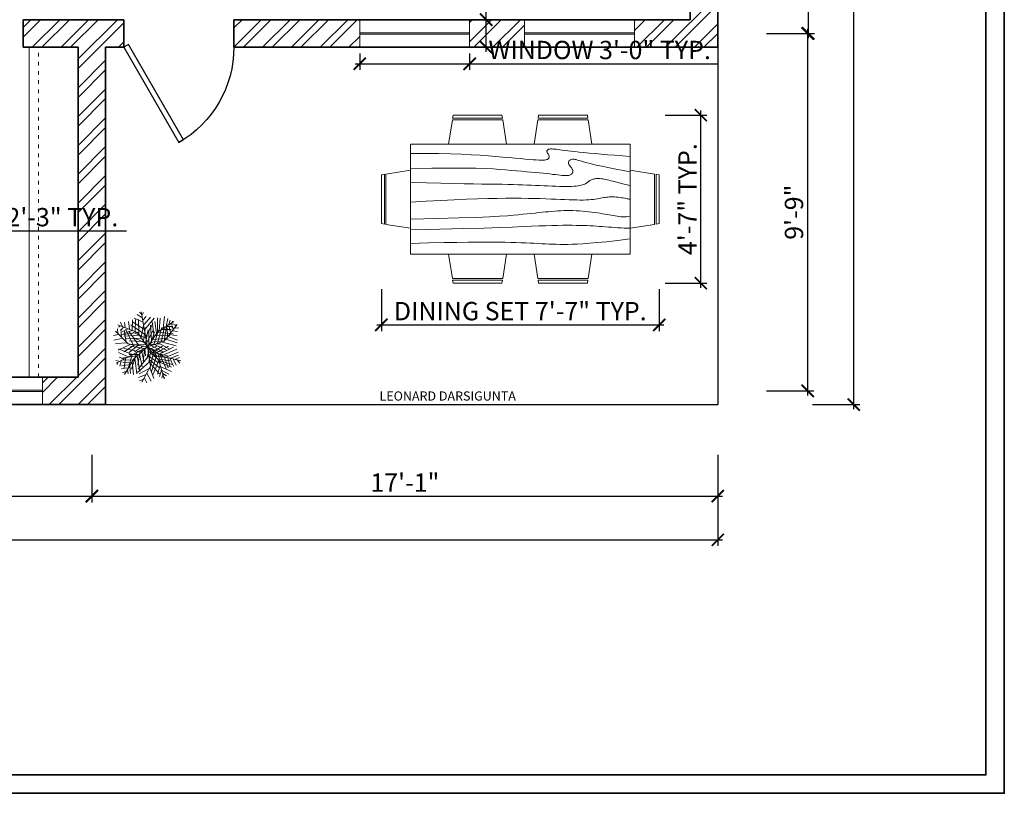
# Model space of a CAD drawing. Units: inches. Extents: x 163 to 947, y 159 to 804.
# Tile 4 of 5: x 625 to 947, y 159 to 412. Entities that reach past the tile are written whole.
import ezdxf

# ---------------------------------------------------------------- set-up
doc = ezdxf.new("R2010")
doc.units = ezdxf.units.IN
doc.linetypes.add('ACAD_ISO03W100', pattern=[30, 12, -18])
for name, color, linetype, lineweight in [('A-ANNO-TEXT', 7, 'Continuous', 18), ('A-ANNO-TTLB', 7, 'Continuous', 35), ('A-FLOR-CASE', 7, 'Continuous', 18), ('A-FLOR-CASE-OVHD', 7, 'ACAD_ISO03W100', 18), ('A-FLOR-OTLN', 7, 'Continuous', 25), ('Dimensions', 7, 'Continuous', 18), ('Doors', 160, 'Continuous', 25), ('Furniture', 40, 'Continuous', 18), ('Greenary  Plants', 100, 'Continuous', 13), ('Wall Hatch', 214, 'Continuous', 13), ('Walls', 222, 'Continuous', 35), ('Windows', 132, 'Continuous', 18)]:
    doc.layers.add(name, color=color, linetype=linetype, lineweight=lineweight)
doc.styles.get("Standard").update_dxf_attribs({"font": 'arial.ttf'})
doc.dimstyles.new('ISO-25', dxfattribs={"dimtxt": 6, "dimasz": 4, "dimexe": 2, "dimexo": 2, "dimtad": 1, "dimdec": 1, "dimlunit": 3, "dimtxsty": 'Standard', "dimblk": 'ARCHTICK', "dimcen": 0, "dimdle": 1.5, "dimadec": 0, "dimazin": 0, "dimtfac": 1, "dimtdec": 1, "dimtmove": 0, "dimatfit": 3, "dimfxl": 13.5, "dimfxlon": 1, "dimarcsym": 0})

# ---------------------------------------------------------------- blocks, each defined once
blk = doc.blocks.new('_ArchTick')
at = {"color": 0, "linetype": 'ByBlock', "const_width": 0.15}
blk.add_lwpolyline([(-0.5, -0.5), (0.5, 0.5)], dxfattribs=at)
blk = doc.blocks.new('*D10')
at = {"layer": 'Dimensions', "color": 0, "lineweight": -2, "transparency": 16777216}
for p, q in [((869.75, 517.32), (885.25, 517.32)), ((883.25, 518.82), (883.25, 405.78)), ((869.75, 407.28), (885.25, 407.28))]:
    blk.add_line(p, q, dxfattribs=at)
at = {"layer": 'Dimensions', "color": 0, "lineweight": -2, "transparency": 16777216, "xscale": 4, "yscale": 4, "zscale": 4}
for p, rotation in [((883.25, 517.32), 90), ((883.25, 407.28), 270)]:
    blk.add_blockref('_ArchTick', p, dxfattribs=dict(at, rotation=rotation))
at = {"layer": 'Dimensions', "color": 0, "transparency": 16777216, "insert": (879.57, 462.3), "char_height": 6, "attachment_point": 5, "rotation": 90}
blk.add_mtext('9\'-2"', dxfattribs=at)
blk = doc.blocks.new('*D11')
at = {"layer": 'Dimensions', "color": 0, "lineweight": -2, "transparency": 16777216}
for p, q in [((869.53, 407.28), (885.03, 407.28)), ((883.03, 408.78), (883.03, 288.78)), ((869.53, 290.28), (885.03, 290.28))]:
    blk.add_line(p, q, dxfattribs=at)
at = {"layer": 'Dimensions', "color": 0, "lineweight": -2, "transparency": 16777216, "xscale": 4, "yscale": 4, "zscale": 4}
for p, rotation in [((883.03, 407.28), 90), ((883.03, 290.28), 270)]:
    blk.add_blockref('_ArchTick', p, dxfattribs=dict(at, rotation=rotation))
at = {"layer": 'Dimensions', "color": 0, "transparency": 16777216, "insert": (879.34, 348.78), "char_height": 6, "attachment_point": 5, "rotation": 90}
blk.add_mtext('9\'-9"', dxfattribs=at)
blk = doc.blocks.new('*D13')
at = {"layer": 'Dimensions', "color": 0, "lineweight": -2, "transparency": 16777216}
for p, q in [((443.62, 269.28), (443.62, 253.78)), ((648.62, 269.28), (648.62, 253.78)), ((442.12, 255.78), (650.12, 255.78))]:
    blk.add_line(p, q, dxfattribs=at)
at = {"layer": 'Dimensions', "color": 0, "lineweight": -2, "transparency": 16777216, "xscale": 4, "yscale": 4, "zscale": 4, "rotation": 180}
blk.add_blockref('_ArchTick', (443.62, 255.78), dxfattribs=at)
at = {"layer": 'Dimensions', "color": 0, "lineweight": -2, "transparency": 16777216, "xscale": 4, "yscale": 4, "zscale": 4}
blk.add_blockref('_ArchTick', (648.62, 255.78), dxfattribs=at)
at = {"layer": 'Dimensions', "color": 0, "transparency": 16777216, "insert": (546.12, 259.41), "char_height": 6, "attachment_point": 5}
blk.add_mtext('17\'-1"', dxfattribs=at)
blk = doc.blocks.new('*D14')
at = {"layer": 'Dimensions', "color": 0, "lineweight": -2, "transparency": 16777216}
for p, q in [((648.62, 269.35), (648.62, 253.85)), ((853.62, 269.35), (853.62, 253.85)), ((647.12, 255.85), (855.12, 255.85))]:
    blk.add_line(p, q, dxfattribs=at)
at = {"layer": 'Dimensions', "color": 0, "lineweight": -2, "transparency": 16777216, "xscale": 4, "yscale": 4, "zscale": 4, "rotation": 180}
blk.add_blockref('_ArchTick', (648.62, 255.85), dxfattribs=at)
at = {"layer": 'Dimensions', "color": 0, "lineweight": -2, "transparency": 16777216, "xscale": 4, "yscale": 4, "zscale": 4}
blk.add_blockref('_ArchTick', (853.62, 255.85), dxfattribs=at)
at = {"layer": 'Dimensions', "color": 0, "transparency": 16777216, "insert": (751.12, 259.48), "char_height": 6, "attachment_point": 5}
blk.add_mtext('17\'-1"', dxfattribs=at)
blk = doc.blocks.new('*U23')
for p, q in [((-36, 0), (-36, 6)), ((0, 0), (0, 6))]:
    blk.add_line(p, q)
blk.add_lwpolyline([(0, 0), (-18, -31.18), (-19.52, -30.3), (-1.52, 0.88)], close=True)
blk.add_arc((0, 0), 36, 180, 240)
blk = doc.blocks.new('Dining Set - 36 x 72 in.')
for p, q in [((-22.2343, 26.00059), (-23.4847, 17.99762)), ((-22.2304, 26), (-5.7608, 26)), ((-22, 27.5), (-22.1562, 26.50042)), ((-5.8416, 26.5), (-22.1534, 26.5)), ((-22, 27.5), (-6, 27.5)), ((-5.8437, 26.49966), (-6, 27.5)), ((-4.5152, 17.99762), (-5.7655, 25.99926)), ((5.7657, 26.00059), (4.5153, 17.99762)), ((5.7696, 26), (22.2392, 26)), ((6, 27.5), (5.8438, 26.50042)), ((22.1584, 26.5), (5.8466, 26.5)), ((6, 27.5), (22, 27.5)), ((22.1563, 26.49966), (22, 27.5)), ((23.4848, 17.99762), (22.2345, 25.99926)), ((36, 18), (-36, 18)), ((-36, 18), (-36, -18)), ((36, -18), (36, 18)), ((-45.5, 8), (-44.5004, 8.15617)), ((-45.5, 8), (-45.5, -8)), ((-44.5, -8.15843), (-44.5, 8.15338)), ((-44.0006, 8.23428), (-35.9976, 9.48474)), ((-44, 8.23041), (-44, -8.23915)), ((44.0006, 8.23428), (35.9976, 9.48474)), ((44, 8.23041), (44, -8.23915)), ((44.5, -8.15843), (44.5, 8.15338)), ((45.5, 8), (44.5005, 8.15617)), ((45.5, 8), (45.5, -8)), ((-44.4997, -8.15631), (-45.5, -8)), ((-35.9976, -9.48476), (-43.9993, -8.2345)), ((35.9976, -9.48476), (43.9993, -8.2345)), ((44.4997, -8.15631), (45.5, -8)), ((-36, -18), (36, -18)), ((-22.2343, -26.0006), (-23.4847, -17.99762)), ((-4.5152, -17.99762), (-5.7655, -25.99928)), ((5.7657, -26.0006), (4.5153, -17.99762)), ((23.4848, -17.99762), (22.2345, -25.99928)), ((-22.2304, -26), (-5.7608, -26)), ((-22, -27.5), (-22.1562, -26.50044)), ((-5.8416, -26.5), (-22.1534, -26.5)), ((-22, -27.5), (-6, -27.5)), ((-5.8437, -26.49967), (-6, -27.5)), ((5.7696, -26), (22.2392, -26)), ((6, -27.5), (5.8438, -26.50044)), ((22.1584, -26.5), (5.8466, -26.5)), ((6, -27.5), (22, -27.5)), ((22.1563, -26.49967), (22, -27.5))]:
    blk.add_line(p, q)
for points in [[(-36, 15), (-31.1772, 14.97754), (-26.8079, 14.91406), (-22.8538, 14.81543), (-19.276, 14.6875), (-16.0362, 14.53613), (-13.0957, 14.36718), (-10.4159, 14.18652), (-7.9583, 14), (-5.6904, 13.81315), (-3.6035, 13.63021), (-1.6954, 13.45508), (0.0365, 13.29166), (1.5945, 13.14388), (2.9811, 13.01562), (4.1988, 12.9108), (5.25, 12.83333), (6.1393, 12.78613), (6.8802, 12.76823), (7.4883, 12.77767), (7.9792, 12.8125), (8.3685, 12.87077), (8.6719, 12.95052), (8.9049, 13.0498), (9.0833, 13.16666), (9.2205, 13.29899), (9.3216, 13.44401), (9.3895, 13.59879), (9.4271, 13.76041), (9.4373, 13.92594), (9.4232, 14.09245), (9.3875, 14.257), (9.3333, 14.41666), (9.2638, 14.56917), (9.1836, 14.71484), (9.0975, 14.85465), (9.0104, 14.98958), (8.9272, 15.1206), (8.8529, 15.2487), (8.7922, 15.37483), (8.75, 15.5), (8.7305, 15.62467), (8.7344, 15.74739), (8.7617, 15.86621), (8.8125, 15.97916), (8.8867, 16.08431), (8.9844, 16.17968), (9.1055, 16.26334), (9.25, 16.33333), (9.4189, 16.38802), (9.6172, 16.42708), (9.8506, 16.45052), (10.125, 16.45833), (10.4463, 16.45052), (10.8203, 16.42708), (11.2529, 16.38802), (11.75, 16.33333), (12.3184, 16.26318), (12.9694, 16.17838), (13.7151, 16.07991), (14.5677, 15.96875), (15.5395, 15.84586), (16.6426, 15.71224), (17.8893, 15.56884), (19.2917, 15.41666), (20.859, 15.25667), (22.5879, 15.08984), (24.4721, 14.91715), (26.5052, 14.73958), (28.6809, 14.5581), (30.9929, 14.3737), (33.4347, 14.18733), (36, 14)], [(-36, 10), (-28.9766, 10.14274), (-23.1725, 10.20442), (-18.4241, 10.19775), (-14.5677, 10.13541), (-11.4399, 10.03011), (-8.877, 9.89453), (-6.7154, 9.74137), (-4.7917, 9.58333), (-2.9698, 9.43082), (-1.2246, 9.28515), (0.4415, 9.14534), (2.026, 9.01041), (3.5266, 8.87939), (4.9408, 8.7513), (6.266, 8.62516), (7.5, 8.5), (8.6411, 8.37549), (9.6914, 8.2539), (10.6538, 8.13818), (11.5312, 8.03125), (12.3267, 7.93603), (13.043, 7.85547), (13.6831, 7.79248), (14.25, 7.75), (14.7471, 7.7303), (15.1797, 7.73307), (15.5537, 7.75732), (15.875, 7.80208), (16.1494, 7.86637), (16.3828, 7.94922), (16.5811, 8.04964), (16.75, 8.16666), (16.8944, 8.29915), (17.0143, 8.44531), (17.1089, 8.60319), (17.1771, 8.77083), (17.218, 8.94629), (17.2305, 9.1276), (17.2137, 9.31282), (17.1667, 9.5), (17.0895, 9.6875), (16.987, 9.875), (16.8649, 10.0625), (16.7292, 10.25), (16.5856, 10.4375), (16.4401, 10.625), (16.2985, 10.8125), (16.1667, 11), (16.05, 11.18733), (15.9518, 11.3737), (15.8752, 11.5581), (15.8229, 11.73958), (15.798, 11.91715), (15.8034, 12.08984), (15.842, 12.25667), (15.9167, 12.41666), (16.0295, 12.56836), (16.1784, 12.70833), (16.3605, 12.83268), (16.5729, 12.9375), (16.8127, 13.01888), (17.0768, 13.07291), (17.3625, 13.0957), (17.6667, 13.08333), (17.9894, 13.03312), (18.3418, 12.94726), (18.7382, 12.82918), (19.1927, 12.68229), (19.7195, 12.51001), (20.3327, 12.31575), (21.0465, 12.10294), (21.875, 11.875), (22.8357, 11.63354), (23.959, 11.37304), (25.2786, 11.08618), (26.8282, 10.76562), (28.6414, 10.40405), (30.752, 9.99414), (33.1936, 9.52856), (36, 9)], [(-36, 5.5), (-30.7157, 5.3348), (-26.069, 5.20963), (-21.9946, 5.11767), (-18.4271, 5.05208), (-15.3009, 5.00602), (-12.5508, 4.97265), (-10.1112, 4.94515), (-7.9167, 4.91666), (-5.909, 4.88167), (-4.0586, 4.83984), (-2.3429, 4.79215), (-0.7396, 4.73958), (0.7739, 4.6831), (2.22, 4.6237), (3.6213, 4.56233), (5, 4.5), (6.373, 4.43782), (7.7344, 4.3776), (9.0723, 4.32129), (10.375, 4.27083), (11.6309, 4.22819), (12.8281, 4.19531), (13.9551, 4.17415), (15, 4.16666), (15.954, 4.17448), (16.819, 4.19791), (17.6001, 4.23698), (18.3021, 4.29166), (18.9299, 4.36198), (19.4883, 4.44791), (19.9823, 4.54948), (20.4167, 4.66666), (20.7969, 4.79899), (21.1302, 4.94401), (21.4245, 5.09879), (21.6875, 5.26041), (21.9271, 5.42594), (22.1511, 5.59245), (22.3672, 5.757), (22.5834, 5.91666), (22.8065, 6.06868), (23.0404, 6.21093), (23.2879, 6.34147), (23.5521, 6.45833), (23.8358, 6.55957), (24.142, 6.64323), (24.4735, 6.70735), (24.8334, 6.75), (25.2235, 6.76969), (25.642, 6.76692), (26.0858, 6.74267), (26.5521, 6.69791), (27.0379, 6.63362), (27.5404, 6.55078), (28.0565, 6.45036), (28.5834, 6.33333), (29.1242, 6.19987), (29.7071, 6.04687), (30.3661, 5.87044), (31.1354, 5.66666), (32.0493, 5.43164), (33.142, 5.16146), (34.4475, 4.85221), (36, 4.5)], [(-36, -1), (-30.7915, -0.6591), (-26.0195, -0.38216), (-21.6519, -0.16284), (-17.6563, 0.00521), (-14.0005, 0.12833), (-10.6523, 0.21289), (-7.5796, 0.26522), (-4.75, 0.29166), (-2.134, 0.29793), (0.2878, 0.28711), (2.5317, 0.26163), (4.6146, 0.22396), (6.5529, 0.17651), (8.3633, 0.12174), (10.0623, 0.06209), (11.6667, 0), (13.1899, -0.06201), (14.6341, -0.1211), (15.9982, -0.17432), (17.2813, -0.21875), (18.4823, -0.25147), (19.6003, -0.26953), (20.6343, -0.27002), (21.5834, -0.25), (22.4481, -0.20768), (23.2357, -0.14584), (23.9549, -0.06836), (24.6146, 0.02083), (25.2235, 0.11784), (25.7904, 0.21875), (26.3241, 0.31966), (26.8334, 0.41666), (27.3265, 0.50618), (27.8099, 0.58593), (28.2894, 0.65397), (28.7709, 0.70833), (29.2601, 0.74707), (29.763, 0.76823), (30.2855, 0.76985), (30.8334, 0.75), (31.4088, 0.70784), (31.9994, 0.64713), (32.589, 0.57275), (33.1615, 0.48958), (33.7008, 0.4025), (34.1908, 0.3164), (34.6153, 0.23616), (34.9584, 0.16666), (35.2099, 0.11165), (35.3848, 0.07031), (35.504, 0.04069), (35.5886, 0.02083), (35.6594, 0.00879), (35.7377, 0.0026), (35.8442, 0.00032), (36, 0)], [(-36, -6.5), (-27.1843, -6.31267), (-20.084, -6.1263), (-14.469, -5.9419), (-10.1094, -5.76042), (-6.7752, -5.58285), (-4.2363, -5.41016), (-2.2629, -5.24333), (-0.625, -5.08334), (0.8708, -4.93099), (2.2715, -4.78646), (3.5872, -4.64974), (4.8281, -4.52084), (6.0046, -4.39974), (7.127, -4.28646), (8.2053, -4.18099), (9.25, -4.08334), (10.2705, -3.99382), (11.2734, -3.91407), (12.2647, -3.84603), (13.25, -3.79167), (14.2354, -3.75293), (15.2266, -3.73177), (16.2295, -3.73015), (17.25, -3.75), (18.2912, -3.79248), (19.3451, -3.85547), (20.4009, -3.93604), (21.4479, -4.03125), (22.4754, -4.13819), (23.4727, -4.25391), (24.4289, -4.37549), (25.3334, -4.5), (26.1785, -4.62492), (26.9694, -4.74935), (27.7145, -4.87281), (28.4219, -4.99479), (29.1, -5.11483), (29.7572, -5.23242), (30.4016, -5.34709), (31.0417, -5.45834), (31.6837, -5.56437), (32.3262, -5.65821), (32.9658, -5.73153), (33.599, -5.77604), (34.2224, -5.78345), (34.8327, -5.74545), (35.4264, -5.65373), (36, -5.5)], [(-36, -10), (-26.4022, -9.81299), (-18.4675, -9.62891), (-11.9839, -9.45069), (-6.7396, -9.28125), (-2.5226, -9.12354), (0.8789, -8.98047), (3.6769, -8.85498), (6.0833, -8.75), (8.2767, -8.66765), (10.3021, -8.60677), (12.1712, -8.56543), (13.8958, -8.54167), (15.4876, -8.53353), (16.9583, -8.53907), (18.3197, -8.55632), (19.5834, -8.58334), (20.7616, -8.61841), (21.8685, -8.66081), (22.9188, -8.71004), (23.9271, -8.76563), (24.9081, -8.82707), (25.8763, -8.89388), (26.8465, -8.96558), (27.8334, -9.04167), (28.8474, -9.12118), (29.8828, -9.20117), (30.93, -9.27824), (31.9792, -9.34896), (33.0205, -9.40991), (34.0443, -9.45768), (35.0407, -9.48885), (36, -9.5)], [(-36, -14.5), (-30.0881, -14.33513), (-25.0332, -14.21224), (-20.7312, -14.12647), (-17.0781, -14.07292), (-13.97, -14.04671), (-11.3027, -14.04297), (-8.9724, -14.05681), (-6.875, -14.08334), (-4.9224, -14.11833), (-3.0905, -14.16016), (-1.3709, -14.20785), (0.2448, -14.26042), (1.7647, -14.3169), (3.1973, -14.3763), (4.5507, -14.43767), (5.8333, -14.5), (7.0554, -14.5621), (8.235, -14.62175), (9.3922, -14.67652), (10.5469, -14.72396), (11.7192, -14.76164), (12.929, -14.78711), (14.1965, -14.79794), (15.5417, -14.79167), (16.9933, -14.76424), (18.6152, -14.70508), (20.4804, -14.60197), (22.6615, -14.44271), (25.2312, -14.21509), (28.2624, -13.9069), (31.8277, -13.50594), (36, -13)]]:
    blk.add_lwpolyline(points)
blk = doc.blocks.new('*U54')
for p, q in [((-8.737, 47.138), (-17.069, 52.711)), ((-10.186, 53.64), (-13.084, 55.962)), ((0, 0), (-10.5, 57)), ((-9.099, 51.782), (-6.563, 55.962)), ((-7.65, 43.423), (-2.578, 49.46)), ((-3.665, 19.273), (-27.574, 35.527)), ((-5.114, 28.097), (-24.676, 40.636)), ((-7.288, 39.707), (-21.778, 46.673)), ((-5.839, 35.992), (4.667, 48.067)), ((-5.114, 27.632), (10.463, 46.673)), ((-2.941, 16.486), (8.652, 37.85)), ((22.055, 7.198), (27.489, 32.277)), ((27, 9), (48, 36)), ((27.127, 9.056), (31.112, 35.992)), ((35.096, 32.741), (37.27, 22.524)), ((38.719, 34.134), (41.979, 28.561)), ((44.153, 36.456), (45.239, 32.741)), ((-47.498, 19.737), (-55.83, 18.344)), ((-31.5, 4.5), (-52.5, 25.5)), ((-48.585, 21.131), (-49.309, 29.026)), ((-43.513, 28.561), (-42.427, 15.558)), ((-38.442, 26.239), (-34.819, 7.663)), ((-35.544, 28.097), (-24.314, 3.947)), ((-14.533, 2.09), (-30.834, 25.31)), ((-24.314, 23.917), (-2.941, 13.7)), ((-1.129, 6.734), (9.014, 26.704)), ((3.942, 1.625), (11.187, 24.381)), ((10.101, 3.483), (17.708, 26.239)), ((16.259, 5.805), (23.142, 31.348)), ((31.836, 30.883), (32.561, 16.486)), ((33.285, 16.486), (48.862, 10.913)), ((36.183, 19.737), (48.137, 17.88)), ((40.53, 25.775), (48.862, 24.846)), ((43.791, 29.954), (51.036, 30.883)), ((-40.615, 13.7), (-55.105, 10.913)), ((-33.37, 6.269), (-52.207, 5.34)), ((-28.299, 3.483), (-47.86, -5.805)), ((-21.416, 3.018), (-38.079, -8.128)), ((0, 0), (-31.5, 4.5)), ((-15.982, 2.09), (-30.11, -9.521)), ((0, 0), (-22.5, -19.5)), ((-6.563, 1.161), (-21.416, -8.128)), ((-20.691, 13.7), (-1.129, 4.876)), ((0, 0), (27, 9)), ((0, 0), (18, -22.5)), ((6.478, 1.625), (26.04, -8.592)), ((11.187, 3.483), (30.749, -5.805)), ((18.07, 5.805), (35.096, -3.483)), ((24.229, 7.663), (46.688, 1.625)), ((29.662, 12.307), (48.137, 6.269)), ((-17.431, -15.094), (-42.789, -18.809)), ((-15.257, -12.772), (-30.11, -12.772)), ((-6.563, -5.805), (-19.967, -9.985)), ((-17.069, -15.094), (-12.721, -40.172)), ((-13.446, -11.378), (-8.737, -32.741)), ((-9.461, -8.592), (-6.201, -23.453)), ((-4.752, -3.483), (-3.665, -14.629)), ((2.493, -3.019), (-1.491, -20.202)), ((1.769, -2.555), (24.229, -9.521)), ((5.029, -6.27), (2.131, -25.775)), ((9.014, -11.378), (3.58, -35.992)), ((7.565, -9.056), (32.198, -14.629)), ((12.274, -15.094), (36.907, -18.809)), ((-28.299, -29.026), (-42.789, -31.348)), ((-24.314, -21.596), (-42.427, -22.06)), ((-26.849, -26.24), (-40.253, -25.775)), ((-22.5, -19.5), (-37.5, -45)), ((-29.023, -30.884), (-27.936, -43.887)), ((-25.038, -23.918), (-22.865, -45.281)), ((-20.691, -18.345), (-17.793, -44.352)), ((14.085, -16.951), (6.478, -40.172)), ((18.07, -22.524), (8.289, -45.745)), ((20.244, -30.419), (15.897, -44.816)), ((16.259, -19.738), (36.183, -22.989)), ((18, -22.5), (27, -52.5)), ((18.433, -22.524), (40.53, -29.026)), ((19.157, -25.311), (38.719, -33.206)), ((-30.834, -34.135), (-42.427, -35.528)), ((-34.457, -39.708), (-40.978, -42.494)), ((-32.646, -36.921), (-31.921, -44.352)), ((22.78, -37.85), (19.519, -48.532)), ((21.331, -32.741), (39.081, -40.636)), ((22.78, -38.314), (34.372, -44.816)), ((24.591, -45.745), (23.142, -50.854)), ((24.591, -43.423), (30.749, -47.603)), ((26.764, -49.925), (28.213, -50.854))]:
    blk.add_line(p, q)
blk = doc.blocks.new('*D58')
at = {"layer": 'Dimensions', "color": 0, "lineweight": -2, "transparency": 16777216}
for p, q in [((262.64, 255.02), (262.64, 239.52)), ((853.62, 255.02), (853.62, 239.52)), ((261.14, 241.52), (855.12, 241.52))]:
    blk.add_line(p, q, dxfattribs=at)
at = {"layer": 'Dimensions', "color": 0, "lineweight": -2, "transparency": 16777216, "xscale": 4, "yscale": 4, "zscale": 4, "rotation": 180}
blk.add_blockref('_ArchTick', (262.64, 241.52), dxfattribs=at)
at = {"layer": 'Dimensions', "color": 0, "lineweight": -2, "transparency": 16777216, "xscale": 4, "yscale": 4, "zscale": 4}
blk.add_blockref('_ArchTick', (853.62, 241.52), dxfattribs=at)
at = {"layer": 'Dimensions', "color": 0, "transparency": 16777216, "insert": (558.13, 245.21), "char_height": 6, "attachment_point": 5}
blk.add_mtext('49\'-3"', dxfattribs=at)
blk = doc.blocks.new('*D59')
at = {"layer": 'Dimensions', "color": 0, "lineweight": -2, "transparency": 16777216}
for p, q in [((884.65, 722.73), (900.15, 722.73)), ((898.15, 284.27), (898.15, 724.23)), ((884.65, 285.77), (900.15, 285.77))]:
    blk.add_line(p, q, dxfattribs=at)
at = {"layer": 'Dimensions', "color": 0, "lineweight": -2, "transparency": 16777216, "xscale": 4, "yscale": 4, "zscale": 4}
for p, rotation in [((898.15, 722.73), 90), ((898.15, 285.77), 270)]:
    blk.add_blockref('_ArchTick', p, dxfattribs=dict(at, rotation=rotation))
at = {"layer": 'Dimensions', "color": 0, "transparency": 16777216, "insert": (894.46, 504.25), "char_height": 6, "attachment_point": 5, "rotation": 90}
blk.add_mtext('36\'-5"', dxfattribs=at)
blk = doc.blocks.new('WIN-36IN')
for p, q in [((0, 9.03), (0, 0)), ((35.98, 9.03), (35.98, 0)), ((0, 4.76), (35.98, 4.76)), ((0, 4.26), (35.98, 4.26))]:
    blk.add_line(p, q)
blk = doc.blocks.new('*D64')
at = {"layer": 'Dimensions', "color": 0, "lineweight": -2, "transparency": 16777216}
for p, q in [((736.35, 400.77), (736.35, 395.37)), ((772.33, 400.77), (772.33, 395.37)), ((734.85, 397.37), (772.33, 397.37)), ((772.33, 397.37), (853.51, 397.37))]:
    blk.add_line(p, q, dxfattribs=at)
at = {"layer": 'Dimensions', "color": 0, "lineweight": -2, "transparency": 16777216, "xscale": 4, "yscale": 4, "zscale": 4, "rotation": 180}
blk.add_blockref('_ArchTick', (736.35, 397.37), dxfattribs=at)
at = {"layer": 'Dimensions', "color": 0, "lineweight": -2, "transparency": 16777216, "xscale": 4, "yscale": 4, "zscale": 4}
blk.add_blockref('_ArchTick', (772.33, 397.37), dxfattribs=at)
at = {"layer": 'Dimensions', "color": 0, "transparency": 16777216, "insert": (814.92, 401.1), "char_height": 6, "attachment_point": 5}
blk.add_mtext('WINDOW 3\'-0" TYP.', dxfattribs=at)
blk = doc.blocks.new('*D65')
at = {"layer": 'Dimensions', "color": 0, "lineweight": -2, "transparency": 16777216}
for p, q in [((777.73, 411.79), (777.73, 453.62)), ((774.33, 411.79), (779.73, 411.79)), ((777.73, 401.27), (777.73, 411.79)), ((774.33, 402.77), (779.73, 402.77))]:
    blk.add_line(p, q, dxfattribs=at)
at = {"layer": 'Dimensions', "color": 0, "lineweight": -2, "transparency": 16777216, "xscale": 4, "yscale": 4, "zscale": 4}
for p, rotation in [((777.73, 411.79), 90), ((777.73, 402.77), 270)]:
    blk.add_blockref('_ArchTick', p, dxfattribs=dict(at, rotation=rotation))
at = {"layer": 'Dimensions', "color": 0, "transparency": 16777216, "insert": (774.04, 434.7), "char_height": 6, "attachment_point": 5, "rotation": 90}
blk.add_mtext('0\'-9" TYP.', dxfattribs=at)
blk = doc.blocks.new('*D68')
at = {"layer": 'Dimensions', "color": 0, "lineweight": -2, "transparency": 16777216}
for p, q in [((743.42, 323.53), (743.42, 309.88)), ((834.42, 323.53), (834.42, 309.88)), ((741.92, 311.88), (835.92, 311.88))]:
    blk.add_line(p, q, dxfattribs=at)
at = {"layer": 'Dimensions', "color": 0, "lineweight": -2, "transparency": 16777216, "xscale": 4, "yscale": 4, "zscale": 4, "rotation": 180}
blk.add_blockref('_ArchTick', (743.42, 311.88), dxfattribs=at)
at = {"layer": 'Dimensions', "color": 0, "lineweight": -2, "transparency": 16777216, "xscale": 4, "yscale": 4, "zscale": 4}
blk.add_blockref('_ArchTick', (834.42, 311.88), dxfattribs=at)
at = {"layer": 'Dimensions', "color": 0, "transparency": 16777216, "insert": (788.92, 315.61), "char_height": 6, "attachment_point": 5}
blk.add_mtext('DINING SET 7\'-7" TYP.', dxfattribs=at)
blk = doc.blocks.new('*D69')
at = {"layer": 'Dimensions', "color": 0, "lineweight": -2, "transparency": 16777216}
for p, q in [((836.42, 380.53), (850.07, 380.53)), ((848.07, 324.03), (848.07, 382.03)), ((836.42, 325.53), (850.07, 325.53))]:
    blk.add_line(p, q, dxfattribs=at)
at = {"layer": 'Dimensions', "color": 0, "lineweight": -2, "transparency": 16777216, "xscale": 4, "yscale": 4, "zscale": 4}
for p, rotation in [((848.07, 380.53), 90), ((848.07, 325.53), 270)]:
    blk.add_blockref('_ArchTick', p, dxfattribs=dict(at, rotation=rotation))
at = {"layer": 'Dimensions', "color": 0, "transparency": 16777216, "insert": (844.45, 353.03), "char_height": 6, "attachment_point": 5, "rotation": 90}
blk.add_mtext('4\'-7" TYP.', dxfattribs=at)
blk = doc.blocks.new('*D70')
at = {"layer": 'Dimensions', "color": 0, "lineweight": -2, "transparency": 16777216}
for p, q in [((551.77, 342.64), (580.27, 342.64)), ((553.27, 340.59), (553.27, 344.64)), ((580.27, 340.59), (580.27, 344.64)), ((580.27, 342.64), (659.97, 342.64))]:
    blk.add_line(p, q, dxfattribs=at)
at = {"layer": 'Dimensions', "color": 0, "lineweight": -2, "transparency": 16777216, "xscale": 4, "yscale": 4, "zscale": 4, "rotation": 180}
blk.add_blockref('_ArchTick', (553.27, 342.64), dxfattribs=at)
at = {"layer": 'Dimensions', "color": 0, "lineweight": -2, "transparency": 16777216, "xscale": 4, "yscale": 4, "zscale": 4}
blk.add_blockref('_ArchTick', (580.27, 342.64), dxfattribs=at)
at = {"layer": 'Dimensions', "color": 0, "transparency": 16777216, "insert": (622.12, 346.37), "char_height": 6, "attachment_point": 5}
blk.add_mtext('ROCKER 2\'-3" TYP.', dxfattribs=at)

msp = doc.modelspace()

# ---------------------------------------------------------------- hatches: boundary and pattern name
at = {"layer": 'Wall Hatch'}
h = msp.add_hatch(dxfattribs=at)
h.set_pattern_fill('ANSI32', color=256, scale=0.7)
h.paths.add_polyline_path([(271.66, 713.71), (308.91, 713.71), (308.91, 722.73), (262.64, 722.73), (262.64, 565.31), (271.66, 565.31), (271.66, 583.27), (310.31, 583.27), (310.31, 587.28), (271.66, 587.28)])
h.paths.add_polyline_path([(357.32, 713.71), (400.68, 713.71), (400.68, 722.73), (344.89, 722.73), (344.89, 713.71), (352.3, 713.71), (352.3, 587.28), (340.31, 587.28), (340.31, 583.27), (387.9, 583.27), (387.9, 580.28), (391.92, 580.28), (391.92, 583.27), (411.3, 583.27), (411.3, 587.28), (357.32, 587.28)])
h.paths.add_polyline_path([(454.65, 722.73), (436.66, 722.73), (436.66, 713.71), (444.3, 713.71), (444.3, 587.28), (441.3, 587.28), (441.3, 583.27), (452.32, 583.27), (452.32, 587.28), (449.32, 587.28), (449.32, 713.71), (454.65, 713.71)])
h.paths.add_polyline_path([(546.44, 722.73), (490.63, 722.73), (490.63, 713.71), (537.42, 713.71), (537.42, 587.28), (482.32, 587.28), (482.32, 583.27), (546.44, 583.27), (546.44, 630.27), (552.44, 630.27), (552.44, 639.3), (546.44, 639.3)])
h.paths.add_polyline_path([(271.66, 529.33), (262.64, 529.33), (262.64, 402.77), (290.54, 402.77), (290.54, 411.79), (271.66, 411.79)])
h.paths.add_polyline_path([(344.49, 408.77), (344.51, 411.79), (326.52, 411.79), (326.52, 402.77), (344.49, 402.77)])
h.paths.add_polyline_path([(528.33, 411.79), (510.34, 411.79), (510.34, 521.35), (546.44, 521.35), (546.44, 525.36), (460.92, 525.36), (460.9, 525.35), (460.9, 521.35), (501.32, 521.35), (501.32, 411.79), (390.5, 411.79), (390.5, 521.35), (430.9, 521.35), (430.9, 525.36), (390.5, 525.36), (390.5, 541.96), (386.49, 541.96), (386.49, 411.79), (380.49, 411.79), (380.49, 402.77), (439.11, 402.77), (439.11, 392.26), (448.14, 392.26), (448.14, 402.77), (528.33, 402.77)])
h.paths.add_polyline_path([(448.14, 356.28), (439.11, 356.28), (439.11, 338.29), (448.14, 338.29)])
h.paths.add_polyline_path([(542.45, 294.79), (448.14, 294.79), (448.14, 302.31), (439.11, 302.31), (439.11, 285.77), (542.45, 285.77)])
h.paths.add_polyline_path([(596.42, 294.79), (578.43, 294.79), (578.43, 285.77), (596.42, 285.77)])
h.paths.add_polyline_path([(653.12, 402.77), (659.11, 402.77), (659.11, 408.77), (659.11, 411.79), (626.1, 411.79), (626.1, 402.77), (644.09, 402.77), (644.09, 294.79), (632.4, 294.79), (632.4, 285.77), (653.12, 285.77)])
h.paths.add_polyline_path([(738.49, 630.27), (844.6, 630.27), (844.6, 603.27), (853.62, 603.27), (853.62, 722.73), (663.29, 722.73), (663.29, 677.29), (672.32, 677.29), (672.32, 713.71), (777.6, 713.71), (777.6, 669.29), (783.62, 669.29), (783.62, 713.71), (844.6, 713.71), (844.6, 636.29), (783.62, 636.29), (783.62, 639.29), (777.6, 639.29), (777.6, 636.29), (672.32, 636.29), (672.32, 645.29), (663.29, 645.29), (663.29, 639.3), (582.43, 639.3), (582.43, 630.27), (643.22, 630.27), (643.22, 624.27), (648.23, 624.27), (648.23, 630.27), (732.47, 630.27), (732.47, 547.43), (648.23, 547.43), (648.23, 594.27), (643.22, 594.27), (643.22, 525.36), (625.17, 525.36), (625.17, 517.34), (648.23, 517.34), (648.23, 541.41), (729.47, 541.41), (729.47, 517.34), (738.49, 517.34)])
h.paths.add_polyline_path([(853.62, 567.29), (844.6, 567.29), (844.6, 489.33), (853.62, 489.33)])
h.paths.add_polyline_path([(853.62, 453.35), (844.6, 453.35), (844.6, 411.79), (826.3, 411.79), (826.3, 402.77), (853.62, 402.77)])
h.paths.add_polyline_path([(790.32, 411.79), (772.33, 411.79), (772.33, 402.77), (790.32, 402.77)])
h.paths.add_polyline_path([(736.35, 411.79), (695.11, 411.79), (695.11, 402.77), (736.35, 402.77)])

# ---------------------------------------------------------------- linework, layer by layer
at = {"layer": 'A-ANNO-TTLB'}
for points in [[(163.29, 792.35), (947.45, 792.35), (947.45, 158.54), (163.29, 158.54)], [(169.29, 786.35), (941.45, 786.35), (941.45, 164.54), (169.29, 164.54)]]:
    msp.add_lwpolyline(points, close=True, dxfattribs=at)
at = {"layer": 'A-FLOR-CASE'}
msp.add_line((628.09, 294.79), (628.09, 402.77), dxfattribs=at)
at = {"layer": 'A-FLOR-CASE-OVHD', "ltscale": 0.1}
msp.add_line((631.09, 294.79), (631.09, 402.77), dxfattribs=at)
at = {"layer": 'A-FLOR-OTLN'}
for p in [(853.62, 402.77), (653.12, 285.77)]:
    msp.add_line(p, (853.62, 285.77), dxfattribs=at)
at = {"layer": 'Walls'}
for p, q in [((853.62, 402.77), (853.62, 722.73)), ((844.6, 411.79), (844.6, 630.27)), ((659.11, 411.79), (626.1, 411.79)), ((626.1, 411.79), (626.1, 402.77)), ((659.11, 411.79), (659.11, 402.77)), ((844.6, 411.79), (695.11, 411.79)), ((695.11, 411.79), (695.11, 402.77)), ((644.09, 402.77), (626.1, 402.77)), ((644.09, 294.79), (644.09, 402.77)), ((653.12, 402.77), (653.12, 285.77)), ((659.11, 402.77), (653.12, 402.77)), ((853.62, 402.77), (695.11, 402.77)), ((448.14, 294.79), (644.09, 294.79)), ((439.11, 285.77), (653.12, 285.77))]:
    msp.add_line(p, q, dxfattribs=at)

# ---------------------------------------------------------------- block references
at = {"layer": 'Doors', "xscale": -1}
msp.add_blockref('*U23', (659.11, 402.77), dxfattribs=at)
at = {"layer": 'Furniture'}
msp.add_blockref('Dining Set - 36 x 72 in.', (788.92, 353.03), dxfattribs=at)
at = {"layer": 'Greenary  Plants', "xscale": 0.2010375495604706, "yscale": 0.2010375495604706, "zscale": 0.2010375495604706, "rotation": 106.8221293867638}
msp.add_blockref('*U54', (666.87, 304.74), dxfattribs=at)
at = {"layer": 'Greenary  Plants', "xscale": 0.2010375495604706, "yscale": 0.2010375495604706, "zscale": 0.2010375495604706}
msp.add_blockref('*U54', (666.87, 304.74), dxfattribs=at)
at = {"layer": 'Windows'}
for p in [(736.35, 402.77), (790.32, 402.77), (596.42, 285.77)]:
    msp.add_blockref('WIN-36IN', p, dxfattribs=at)

# ---------------------------------------------------------------- texts
at = {"layer": 'A-ANNO-TEXT', "insert": (680.86, 290.1), "char_height": 3, "attachment_point": 1}
msp.add_mtext_dynamic_manual_height_columns('\\pxqc;{\\fTimes New Roman|b1|i0|c0|p18;\\T2.7;LEONARD DARSIGUNTA}', width=168.5705, gutter_width=12.5, heights=[0], dxfattribs=at)

# ---------------------------------------------------------------- dimensions: what is measured, and where the dimension line sits
at = {"layer": 'Dimensions'}
for base, p1, p2, picture, middle in [((898.15, 722.73), (853.62, 285.77), (853.62, 722.73), '*D59', (894.46, 504.25)), ((883.25, 407.28), (858.02, 517.32), (858.02, 407.28), '*D10', (879.57, 462.3)), ((883.03, 290.28), (858.02, 407.28), (858.02, 290.28), '*D11', (879.34, 348.78))]:
    dim = msp.add_linear_dim(base=base, p1=p1, p2=p2, angle=90, dimstyle='ISO-25', override={"dimclrd": 0, "dimclre": 0, "dimclrt": 0}, dxfattribs=at)
    dim.commit()
    dim.dimension.update_dxf_attribs({"geometry": picture, "text_midpoint": middle})
for base, p1, p2, angle, text, picture, middle in [((777.73, 411.79), (772.33, 402.77), (772.33, 411.79), 90, '<> TYP.', '*D65', (774.04, 434.7)), ((848.07, 380.53), (834.42, 325.53), (834.42, 380.53), 90, '<> TYP.', '*D69', (844.45, 353.03)), ((580.27, 342.64), (553.27, 338.59), (580.27, 338.59), 360, 'ROCKER <> TYP.', '*D70', (622.12, 346.37))]:
    dim = msp.add_linear_dim(base=base, p1=p1, p2=p2, angle=angle, text=text, dimstyle='ISO-25', override={"dimdec": 1, "dimlfac": 1, "dimrnd": 0, "dimzin": 1, "dimdsep": 46, "dimlunit": 4, "dimfrac": 2}, dxfattribs=at)
    dim.commit()
    dim.dimension.update_dxf_attribs({"geometry": picture, "text_midpoint": middle})
for base, p1, p2, text, picture, middle in [((772.33, 397.37), (736.35, 402.77), (772.33, 402.77), 'WINDOW <> TYP.', '*D64', (814.92, 401.1)), ((834.42, 311.88), (743.42, 325.53), (834.42, 325.53), 'DINING SET <> TYP.', '*D68', (788.92, 315.61))]:
    dim = msp.add_linear_dim(base=base, p1=p1, p2=p2, text=text, dimstyle='ISO-25', override={"dimdec": 1, "dimlfac": 1, "dimrnd": 0, "dimzin": 1, "dimdsep": 46, "dimlunit": 4, "dimfrac": 2}, dxfattribs=at)
    dim.commit()
    dim.dimension.update_dxf_attribs({"geometry": picture, "text_midpoint": middle})
for base, p1, p2, picture, middle in [((853.62, 241.52), (262.64, 285.77), (853.62, 285.77), '*D58', (558.13, 245.21)), ((648.62, 255.78), (443.62, 281.76), (648.62, 281.76), '*D13', (546.12, 259.41)), ((853.62, 255.85), (648.62, 281.76), (853.62, 281.76), '*D14', (751.12, 259.48))]:
    dim = msp.add_linear_dim(base=base, p1=p1, p2=p2, dimstyle='ISO-25', override={"dimclrd": 0, "dimclre": 0, "dimclrt": 0}, dxfattribs=at)
    dim.commit()
    dim.dimension.update_dxf_attribs({"geometry": picture, "text_midpoint": middle})

doc.saveas('drawing.dxf')
